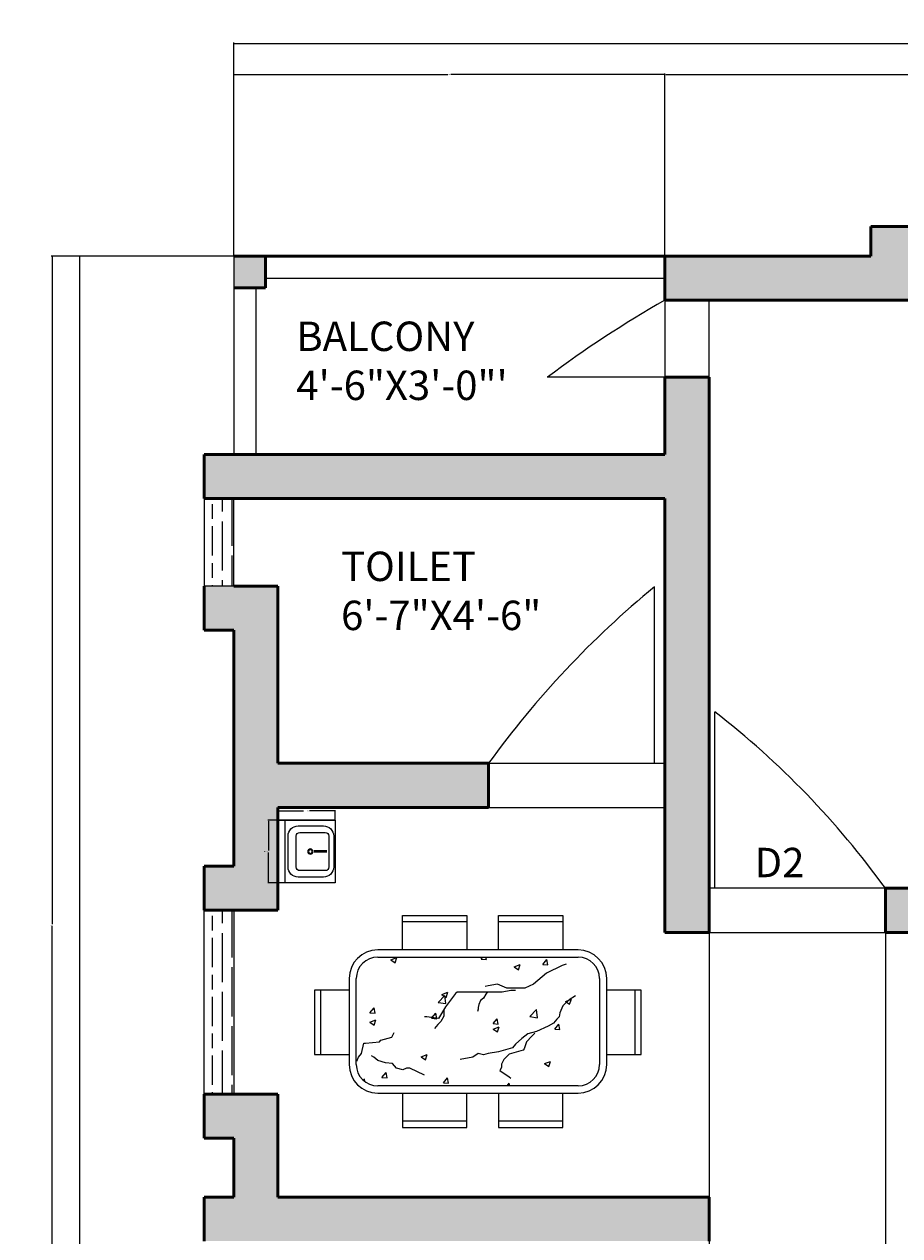
# Model space of a CAD drawing. Units: inches. Extents: x -12 to 604, y -566 to 58.
# Tile 5 of 12: x -12 to 166, y -189 to 58. Entities that reach past the tile are written whole.
import ezdxf

# ---------------------------------------------------------------- set-up
doc = ezdxf.new("R2010")
doc.units = ezdxf.units.IN
doc.header["$MEASUREMENT"] = 0
for name, color, linetype, lineweight in [('A-ANNO-DIMS', 2, 'Continuous', 18), ('A-ANNO-TEXT', 7, 'Continuous', 18), ('A-AREA-IDEN', 7, 'Continuous', 18), ('A-DOOR', 4, 'Continuous', 25), ('A-FLOR-FIXT', 9, 'Continuous', 18), ('A-FLOR-RAIL', 7, 'Continuous', 25), ('A-FURN', 8, 'Continuous', 18), ('A-GLAZ', 82, 'Continuous', 18), ('A-GLAZ-PATT', 82, 'Continuous', 13), ('A-WALL', 7, 'Continuous', 50), ('A-WALL-PATT', 18, 'Continuous', 13)]:
    doc.layers.add(name, color=color, linetype=linetype, lineweight=lineweight)
doc.styles.get("Standard").update_dxf_attribs({"font": 'arial.ttf'})
doc.dimstyles.get("Standard").update_dxf_attribs({"dimtxt": 0.18, "dimasz": 0.18, "dimexe": 0.18, "dimexo": 0.0625, "dimgap": 0.09, "dimtad": 0, "dimtih": 1, "dimtoh": 1, "dimdec": 0, "dimzin": 0, "dimdsep": 46, "dimlunit": 3, "dimtxsty": 'Standard', "dimcen": 0.09, "dimadec": 0, "dimazin": 0, "dimtfac": 1, "dimtdec": 0, "dimtofl": 0, "dimtmove": 0, "dimatfit": 3, "dimfxl": 1, "dimtolj": 1, "dimtzin": 0, "dimarcsym": 0})
pattern_1 = [(90, (0, 0), (6, -4e-16), [10, -2]), (90, (2, -2), (6, -4e-16), [6, -1.5, 3, -1.5]), (90, (4, -5), (6, -4e-16), [10, -2])]

# ---------------------------------------------------------------- blocks, each defined once
blk = doc.blocks.new('М14 600х655')
for p, q in [((-655, 600), (-655, 0)), ((-655, 600), (-655, 0)), ((-655, 0), (-655, 600)), ((0, 600), (-655, 600)), ((0, 525), (-655, 525)), ((0, 0), (0, 600)), ((-596, 388), (-596, 121)), ((-165, 494), (-490, 494)), ((-165, 408), (-490, 408)), ((-59, 121), (-59, 388)), ((-528, 370), (-528, 103)), ((-127, 103), (-127, 370)), ((-334, 87), (-334, 220)), ((-321, 87), (-321, 220)), ((-655, 0), (-655, 0)), ((-655, 0), (-655, 0)), ((-655, 0), (0, 0)), ((-655, 0), (0, 0)), ((-490, 65), (-165, 65)), ((-490, 15), (-165, 15))]:
    blk.add_line(p, q)
for radius in [27.6, 19.3]:
    blk.add_circle((-327, 259), radius)
for centre, radius, start, end in [((-490, 388), 106, 90, 180), ((-490, 370), 38.2, 90, 180), ((-165, 388), 106, 0, 90), ((-165, 370), 38.2, 0, 90), ((-490, 121), 106, 180, 270), ((-490, 103), 38.2, 180, 270), ((-165, 121), 106, 270, 0), ((-165, 103), 38.2, 270, 0)]:
    blk.add_arc(centre, radius, start, end)
blk = doc.blocks.new('*D4')
at = {"layer": 'A-ANNO-DIMS', "color": 0, "lineweight": -2, "transparency": 16777216}
for p, q in [((30.32, 11.2), (30.32, 54.68)), ((30.5, 54.5), (303.81, 54.5)), ((598.14, 54.5), (324.84, 54.5)), ((598.32, 11.2), (598.32, 54.68))]:
    blk.add_line(p, q, dxfattribs=at)
at = {"layer": 'A-ANNO-DIMS', "color": 0, "transparency": 16777216}
for points in [[(30.5, 54.53), (30.5, 54.47), (30.32, 54.5)], [(598.14, 54.53), (598.14, 54.47), (598.32, 54.5)]]:
    blk.add_solid(points, dxfattribs=at)
at = {"layer": 'Defpoints', "color": 0, "transparency": 16777216}
for p in [(598.32, 54.5), (30.32, 11.14), (598.32, 11.14)]:
    blk.add_point(p, dxfattribs=at)
at = {"layer": 'A-ANNO-DIMS', "color": 0, "transparency": 16777216, "insert": (314.32, 54.5), "char_height": 6, "attachment_point": 5}
blk.add_mtext('\\A1;47\'-4"', dxfattribs=at)
blk = doc.blocks.new('*D5')
at = {"layer": 'A-ANNO-DIMS', "color": 0, "lineweight": -2, "transparency": 16777216}
for p, q in [((30.26, 11.14), (-1.3, 11.14)), ((-1.12, 10.96), (-1.12, -233.2)), ((-1.12, -483.68), (-1.12, -239.51)), ((30.26, -483.86), (-1.3, -483.86))]:
    blk.add_line(p, q, dxfattribs=at)
at = {"layer": 'A-ANNO-DIMS', "color": 0, "transparency": 16777216}
for points in [[(-1.15, 10.96), (-1.09, 10.96), (-1.12, 11.14)], [(-1.15, -483.68), (-1.09, -483.68), (-1.12, -483.86)]]:
    blk.add_solid(points, dxfattribs=at)
at = {"layer": 'Defpoints', "color": 0, "transparency": 16777216}
for p in [(30.32, 11.14), (-1.12, -483.86), (30.32, -483.86)]:
    blk.add_point(p, dxfattribs=at)
at = {"layer": 'A-ANNO-DIMS', "color": 0, "transparency": 16777216, "insert": (-1.12, -236.36), "char_height": 6, "attachment_point": 5}
blk.add_mtext('\\A1;41\'-3"', dxfattribs=at)
blk = doc.blocks.new('DINING-TABLE-6-SEAT')
for p, q in [((17.93, 36.25), (17.93, 43.28)), ((17.93, 43.28), (31.08, 43.28)), ((31.08, 43.28), (31.08, 36.25)), ((37.5, 36.25), (37.5, 43.28)), ((37.5, 43.28), (50.64, 43.28)), ((50.64, 43.28), (50.64, 36.25)), ((31.08, 42), (17.93, 42)), ((50.64, 42), (37.5, 42)), ((53.77, 36.25), (12.88, 36.25)), ((12.88, 34.79), (53.77, 34.79)), ((15.53, 34.2), (16.76, 34.67)), ((16.41, 33.61), (16.76, 34.67)), ((34.01, 34.38), (34.34, 34.79)), ((35.05, 34.29), (34.96, 34.79)), ((15.53, 34.2), (16.41, 33.61)), ((34.01, 34.38), (35.05, 34.29)), ((40.72, 32.8), (41.94, 33.27)), ((40.72, 32.8), (41.59, 32.21)), ((41.59, 32.21), (41.95, 33.27)), ((46.57, 33.28), (47.42, 34.29)), ((46.57, 33.28), (47.62, 33.19)), ((50.53, 33.06), (47.35, 31.47)), ((47.62, 33.19), (47.42, 34.29)), ((51.32, 33.37), (50.53, 33.06)), ((7.04, 30.4), (7.04, 12.88)), ((8.5, 12.88), (8.5, 30.4)), ((47.35, 31.47), (44.66, 29.25)), ((58.15, 30.4), (58.15, 12.88)), ((59.61, 12.88), (59.61, 30.4)), ((0, 28.04), (0, 14.9)), ((7.04, 28.04), (0, 28.04)), ((1.29, 14.9), (1.29, 28.04)), ((25.99, 27.15), (27.22, 27.62)), ((28.78, 27.35), (26.71, 24.65)), ((26.87, 26.56), (27.22, 27.62)), ((29.09, 27.66), (28.78, 27.35)), ((38.3, 27.66), (29.09, 27.66)), ((35.45, 28.93), (34.81, 28.77)), ((35.29, 27.67), (34.97, 27.19)), ((37.35, 29.25), (35.45, 28.93)), ((39.26, 28.46), (37.35, 29.25)), ((40.05, 27.98), (38.3, 27.66)), ((42.91, 28.46), (39.26, 28.46)), ((41, 27.98), (40.05, 27.98)), ((44.66, 29.25), (42.91, 28.46)), ((66.65, 28.04), (59.61, 28.04)), ((65.37, 28.04), (65.37, 14.9)), ((66.65, 14.9), (66.65, 28.04)), ((25.21, 25.55), (26.57, 26.98)), ((25.21, 25.55), (26.76, 25.31)), ((25.99, 27.15), (26.87, 26.56)), ((26.76, 25.31), (26.57, 26.98)), ((33.54, 25.13), (33.38, 24.5)), ((33.86, 25.92), (33.54, 25.13)), ((34.49, 26.4), (33.86, 25.92)), ((34.97, 27.19), (34.49, 26.4)), ((50.69, 24.81), (50.05, 23.38)), ((51.96, 26.08), (50.69, 24.81)), ((51.18, 25.74), (52.41, 26.21)), ((51.18, 25.74), (52.05, 25.15)), ((53.23, 26.87), (51.96, 26.08)), ((52.05, 25.15), (52.41, 26.21)), ((11.3, 23.4), (12.14, 24.41)), ((11.3, 23.4), (12.35, 23.31)), ((12.35, 23.31), (12.14, 24.41)), ((22.9, 22.59), (22.42, 22.59)), ((25.28, 22.27), (22.9, 22.59)), ((23.87, 22.3), (24.71, 23.31)), ((23.87, 22.3), (24.91, 22.21)), ((24.92, 22.21), (24.71, 23.31)), ((26.71, 24.65), (25.28, 22.27)), ((26.39, 22.75), (25.76, 21.64)), ((26.39, 24.17), (26.39, 22.75)), ((33.38, 24.18), (33.22, 23.7)), ((33.38, 24.5), (33.38, 24.18)), ((43.91, 22.65), (45.27, 24.08)), ((43.91, 22.65), (45.47, 22.41)), ((45.47, 22.41), (45.27, 24.07)), ((49.9, 22.59), (49.42, 22.11)), ((50.05, 23.38), (49.9, 22.59)), ((11.27, 21.49), (12.5, 21.97)), ((11.27, 21.49), (12.14, 20.91)), ((12.14, 20.91), (12.5, 21.96)), ((25.12, 21), (24.49, 20.21)), ((25.76, 21.64), (25.12, 21)), ((36.44, 21.2), (37.28, 22.21)), ((36.44, 21.2), (37.48, 21.11)), ((36.45, 20.09), (37.68, 20.56)), ((36.45, 20.09), (37.33, 19.5)), ((37.48, 21.11), (37.28, 22.21)), ((37.33, 19.5), (37.68, 20.56)), ((47.67, 20.68), (45.29, 19.57)), ((48.78, 21.32), (47.67, 20.68)), ((49.42, 22.11), (48.78, 21.32)), ((49.01, 20.1), (49.85, 21.11)), ((49.01, 20.1), (50.05, 20.01)), ((50.05, 20.01), (49.85, 21.11)), ((10.36, 17.19), (13.21, 17.51)), ((13.21, 17.51), (13.53, 17.83)), ((13.53, 17.83), (15.76, 18.46)), ((15.76, 18.46), (16.23, 19.41)), ((42.27, 18.15), (41, 17.04)), ((43.54, 19.1), (42.27, 18.15)), ((43.23, 17.51), (42.75, 16.08)), ((44.34, 18.62), (43.23, 17.51)), ((45.29, 19.57), (43.54, 19.1)), ((44.97, 19.26), (44.34, 18.62)), ((0, 14.9), (7.04, 14.9)), ((8.93, 14.34), (9.56, 15.13)), ((9.56, 15.13), (10.04, 17.19)), ((10.04, 17.19), (10.36, 17.19)), ((21.73, 14.44), (22.96, 14.91)), ((22.6, 13.85), (22.96, 14.91)), ((33.38, 15.13), (32.27, 14.34)), ((34.49, 14.82), (33.38, 15.13)), ((35.45, 15.13), (34.49, 14.82)), ((37.51, 15.45), (35.45, 15.13)), ((40.37, 16.24), (37.51, 15.45)), ((39.73, 14.97), (38.62, 13.86)), ((42.59, 15.77), (39.73, 14.97)), ((41, 17.04), (40.37, 16.24)), ((42.75, 16.08), (42.59, 15.77)), ((59.61, 14.9), (66.65, 14.9)), ((8.61, 13.55), (8.93, 14.34)), ((12.11, 14.35), (11.63, 14.66)), ((12.9, 13.71), (12.11, 14.35)), ((14.49, 13.23), (12.9, 13.71)), ((15.92, 13.08), (14.49, 13.23)), ((16.71, 12.12), (15.92, 13.08)), ((21.73, 14.44), (22.6, 13.85)), ((32.27, 14.34), (29.73, 13.86)), ((38.62, 13.86), (38.14, 12.91)), ((38.14, 12.91), (38.14, 12.28)), ((46.91, 13.04), (48.14, 13.51)), ((46.91, 13.04), (47.79, 12.45)), ((47.79, 12.45), (48.14, 13.51)), ((9.93, 9.64), (10.19, 9.91)), ((10.25, 9.37), (10.19, 9.9)), ((13.73, 10.22), (14.57, 11.23)), ((13.73, 10.22), (14.78, 10.13)), ((14.78, 10.13), (14.57, 11.23)), ((17.98, 11.81), (16.71, 12.12)), ((18.77, 12.12), (17.98, 11.81)), ((19.41, 12.12), (18.77, 12.12)), ((22.43, 10.7), (19.41, 12.12)), ((26.3, 9.12), (27.14, 10.13)), ((27.35, 9.03), (27.14, 10.13)), ((38.14, 12.28), (37.83, 11.64)), ((37.83, 11.64), (39.73, 10.37)), ((39.73, 10.37), (40.05, 10.06)), ((53.77, 8.5), (12.88, 8.5)), ((26.3, 9.12), (27.35, 9.03)), ((39.27, 8.5), (39.71, 9.03)), ((39.81, 8.5), (39.71, 9.03)), ((12.88, 7.04), (53.77, 7.04)), ((17.93, 7.04), (17.93, 0)), ((31.08, 0), (31.08, 7.04)), ((37.5, 7.04), (37.5, 0)), ((50.64, 0), (50.64, 7.04)), ((31.08, 1.29), (17.93, 1.29)), ((50.64, 1.29), (37.5, 1.29)), ((17.93, 0), (31.08, 0)), ((37.5, 0), (50.64, 0))]:
    blk.add_line(p, q)
for centre, radius, start, end in [((12.88, 30.4), 5.84, 90, 180), ((12.88, 30.4), 4.38, 90, 180), ((53.77, 30.4), 5.84, 0, 90), ((53.77, 30.4), 4.38, 0, 90), ((12.88, 12.88), 5.84, 180, 270), ((12.88, 12.88), 4.38, 180, 270), ((53.77, 12.88), 4.38, 270, 0), ((53.77, 12.88), 5.84, 270, 0)]:
    blk.add_arc(centre, radius, start, end)
blk = doc.blocks.new('*D27')
at = {"layer": 'A-ANNO-DIMS', "color": 0, "lineweight": -2, "transparency": 16777216}
for p, q in [((39.28, -104), (37.25, -104)), ((37.43, -104.18), (37.43, -110.18)), ((37.43, -116.55), (37.43, -110.55)), ((39.28, -116.73), (37.25, -116.73))]:
    blk.add_line(p, q, dxfattribs=at)
at = {"layer": 'A-ANNO-DIMS', "color": 0, "transparency": 16777216}
for points in [[(37.4, -104.18), (37.46, -104.18), (37.43, -104)], [(37.4, -116.55), (37.46, -116.55), (37.43, -116.73)]]:
    blk.add_solid(points, dxfattribs=at)
at = {"layer": 'Defpoints', "color": 0, "transparency": 16777216}
for p in [(39.34, -104), (37.43, -116.73), (39.34, -116.73)]:
    blk.add_point(p, dxfattribs=at)
at = {"layer": 'A-ANNO-DIMS', "color": 0, "transparency": 16777216, "insert": (37.43, -110.36), "char_height": 0.18, "attachment_point": 5}
blk.add_mtext('\\A1;BASIN 1\'-0 1/2"', dxfattribs=at)
blk = doc.blocks.new('*D28')
at = {"layer": 'A-ANNO-DIMS', "color": 0, "lineweight": -2, "transparency": 16777216}
for p, q in [((39.34, -103.93), (39.34, -101.91)), ((39.52, -102.09), (44.56, -102.09)), ((50.83, -102.09), (45.78, -102.09)), ((51.01, -103.93), (51.01, -101.91))]:
    blk.add_line(p, q, dxfattribs=at)
at = {"layer": 'A-ANNO-DIMS', "color": 0, "transparency": 16777216}
for points in [[(39.52, -102.06), (39.52, -102.12), (39.34, -102.09)], [(50.83, -102.06), (50.83, -102.12), (51.01, -102.09)]]:
    blk.add_solid(points, dxfattribs=at)
at = {"layer": 'Defpoints', "color": 0, "transparency": 16777216}
for p in [(39.34, -102.09), (39.34, -104), (51.01, -104)]:
    blk.add_point(p, dxfattribs=at)
at = {"layer": 'A-ANNO-DIMS', "color": 0, "transparency": 16777216, "insert": (45.17, -102.09), "char_height": 0.18, "attachment_point": 5}
blk.add_mtext('\\A1;0\'-11 1/2"', dxfattribs=at)
blk = doc.blocks.new('*D51')
at = {"layer": 'A-ANNO-DIMS', "color": 0, "lineweight": -2, "transparency": 16777216}
for p, q in [((30.32, 11.2), (30.32, 48.37)), ((30.5, 48.19), (73.99, 48.19)), ((118.14, 48.19), (74.65, 48.19)), ((118.32, 11.2), (118.32, 48.37))]:
    blk.add_line(p, q, dxfattribs=at)
at = {"layer": 'A-ANNO-DIMS', "color": 0, "transparency": 16777216}
for points in [[(30.5, 48.22), (30.5, 48.16), (30.32, 48.19)], [(118.14, 48.22), (118.14, 48.16), (118.32, 48.19)]]:
    blk.add_solid(points, dxfattribs=at)
at = {"layer": 'Defpoints', "color": 0, "transparency": 16777216}
for p in [(118.32, 48.19), (30.32, 11.14), (118.32, 11.14)]:
    blk.add_point(p, dxfattribs=at)
at = {"layer": 'A-ANNO-DIMS', "color": 0, "transparency": 16777216, "insert": (74.32, 48.19), "char_height": 0.18, "attachment_point": 5}
blk.add_mtext('\\A1;7\'-4"', dxfattribs=at)
blk = doc.blocks.new('*D52')
at = {"layer": 'A-ANNO-DIMS', "color": 0, "lineweight": -2, "transparency": 16777216}
for p, q in [((118.32, 11.2), (118.32, 48.37)), ((118.5, 48.19), (198.93, 48.19)), ((280.14, 48.19), (199.71, 48.19)), ((280.32, 11.2), (280.32, 48.37))]:
    blk.add_line(p, q, dxfattribs=at)
at = {"layer": 'A-ANNO-DIMS', "color": 0, "transparency": 16777216}
for points in [[(118.5, 48.22), (118.5, 48.16), (118.32, 48.19)], [(280.14, 48.22), (280.14, 48.16), (280.32, 48.19)]]:
    blk.add_solid(points, dxfattribs=at)
at = {"layer": 'Defpoints', "color": 0, "transparency": 16777216}
for p in [(280.32, 48.19), (118.32, 11.14), (280.32, 11.14)]:
    blk.add_point(p, dxfattribs=at)
at = {"layer": 'A-ANNO-DIMS', "color": 0, "transparency": 16777216, "insert": (199.32, 48.19), "char_height": 0.18, "attachment_point": 5}
blk.add_mtext('\\A1;13\'-6"', dxfattribs=at)
blk = doc.blocks.new('*D54')
at = {"layer": 'A-ANNO-DIMS', "color": 0, "lineweight": -2, "transparency": 16777216}
for p, q in [((30.26, 11.14), (-6.91, 11.14)), ((-6.73, 10.96), (-6.73, -125.18)), ((-6.73, -261.68), (-6.73, -125.54)), ((39.26, -261.86), (-6.91, -261.86))]:
    blk.add_line(p, q, dxfattribs=at)
at = {"layer": 'A-ANNO-DIMS', "color": 0, "transparency": 16777216}
for points in [[(-6.76, 10.96), (-6.7, 10.96), (-6.73, 11.14)], [(-6.76, -261.68), (-6.7, -261.68), (-6.73, -261.86)]]:
    blk.add_solid(points, dxfattribs=at)
at = {"layer": 'Defpoints', "color": 0, "transparency": 16777216}
for p in [(30.32, 11.14), (-6.73, -261.86), (39.32, -261.86)]:
    blk.add_point(p, dxfattribs=at)
at = {"layer": 'A-ANNO-DIMS', "color": 0, "transparency": 16777216, "insert": (-6.73, -125.36), "char_height": 0.18, "attachment_point": 5}
blk.add_mtext('\\A1;22\'-9"', dxfattribs=at)
blk = doc.blocks.new('*D56')
at = {"layer": 'A-ANNO-DIMS', "color": 0, "lineweight": -2, "transparency": 16777216}
for p, q in [((127.32, -117.92), (127.32, -565.59)), ((163.32, -117.92), (163.32, -565.59)), ((127.5, -565.41), (144.99, -565.41)), ((163.14, -565.41), (145.65, -565.41))]:
    blk.add_line(p, q, dxfattribs=at)
at = {"layer": 'A-ANNO-DIMS', "color": 0, "transparency": 16777216}
for points in [[(127.5, -565.38), (127.5, -565.44), (127.32, -565.41)], [(163.14, -565.38), (163.14, -565.44), (163.32, -565.41)]]:
    blk.add_solid(points, dxfattribs=at)
at = {"layer": 'Defpoints', "color": 0, "transparency": 16777216}
for p in [(127.32, -117.86), (163.32, -117.86), (163.32, -565.41)]:
    blk.add_point(p, dxfattribs=at)
at = {"layer": 'A-ANNO-DIMS', "color": 0, "transparency": 16777216, "insert": (145.32, -565.41), "char_height": 0.18, "attachment_point": 5}
blk.add_mtext('\\A1;3\'-0"', dxfattribs=at)

msp = doc.modelspace()

# ---------------------------------------------------------------- hatches: boundary and pattern name
at = {"layer": 'A-GLAZ-PATT'}
h = msp.add_hatch(dxfattribs=at)
h.set_pattern_fill('GOST_WOOD', color=256)
h.set_pattern_definition(pattern_1)
h.paths.add_polyline_path([(30.32, -38.36), (24.32, -38.36), (24.32, -56.22), (30.32, -56.22)])
h = msp.add_hatch(dxfattribs=at)
h.set_pattern_fill('GOST_WOOD', color=256)
h.set_pattern_definition(pattern_1)
h.paths.add_polyline_path([(30.32, -122.36), (24.32, -122.36), (24.32, -159.86), (30.32, -159.86)])
at = {"layer": 'A-WALL-PATT'}
h = msp.add_hatch(color=256, dxfattribs=at)
h.dxf.hatch_style = 1
h.paths.add_polyline_path([(169.32, 11.14), (169.32, 17.14), (160.32, 17.14), (160.32, 11.14), (118.32, 11.14), (118.32, 6.64), (118.32, 2.14), (127.32, 2.14), (169.32, 2.14)])
h.paths.add_polyline_path([(127.32, -13.61), (118.32, -13.61), (118.32, -29.36), (34.82, -29.36), (24.32, -29.36), (24.32, -38.36), (39.32, -38.36), (118.32, -38.36), (118.32, -126.86), (127.32, -126.86), (127.32, -117.86)])
h.paths.add_polyline_path([(82.32, -92.36), (39.32, -92.36), (39.32, -56.22), (30.32, -56.22), (24.32, -56.22), (24.32, -65.22), (30.32, -65.22), (30.32, -113.36), (24.32, -113.36), (24.32, -122.36), (39.32, -122.36), (39.32, -101.36), (82.32, -101.36), (82.32, -96.86)], flags=17)
h.paths.add_polyline_path([(280.32, 11.14), (238.32, 11.14), (238.32, 17.14), (229.32, 17.14), (229.32, 12.64), (229.32, 11.14), (229.32, 2.14), (271.32, 2.14), (271.32, -117.86), (163.32, -117.86), (163.32, -126.86), (271.32, -126.86), (271.32, -189.86), (280.32, -189.86), (280.32, -180.86)])
h.paths.add_polyline_path([(415.32, 17.14), (406.32, 17.14), (406.32, 11.14), (358.32, 11.14), (358.32, -21.86), (367.32, -21.86), (367.32, 2.14), (415.32, 2.14)], flags=17)
h.paths.add_polyline_path([(484.55, -45.86), (448.32, -45.86), (448.32, 2.14), (448.32, 17.14), (439.32, 17.14), (439.32, 12.64), (439.32, 2.14), (439.32, -45.86), (367.32, -45.86), (358.32, -45.86), (358.32, -54.86), (430.32, -54.86), (430.32, -69.59), (430.32, -180.86), (318.82, -180.86), (318.82, -189.86), (318.82, -331.86), (327.82, -331.86), (327.82, -189.86), (439.32, -189.86), (439.32, -180.86), (439.32, -54.86), (483.5, -54.86), (484.55, -54.86)])
h.paths.add_polyline_path([(529.32, 11.14), (481.32, 11.14), (481.32, 17.14), (472.32, 17.14), (472.32, 12.64), (472.32, 2.14), (520.32, 2.14), (520.32, -21.86), (529.32, -21.86)])
h.paths.add_polyline_path([(598.32, -45.86), (582.42, -45.86), (582.42, -50.36), (582.42, -54.86), (589.32, -54.86), (589.32, -99.86), (598.32, -99.86), (604.32, -99.86), (604.32, -90.86), (598.32, -90.86)])
h.paths.add_polyline_path([(598.32, -168.86), (604.32, -168.86), (604.32, -159.86), (589.32, -159.86), (589.32, -180.86), (477.32, -180.86), (477.32, -189.86), (477.32, -259.86), (486.32, -259.86), (486.32, -189.86), (589.32, -189.86), (589.32, -204.86), (598.32, -204.86), (604.32, -204.86), (604.32, -195.86), (598.32, -195.86)])
h.paths.add_polyline_path([(598.32, -244.86), (604.32, -244.86), (604.32, -235.86), (598.32, -235.86), (589.32, -235.86), (589.32, -250.86), (522.32, -250.86), (522.32, -259.86), (589.32, -259.86), (589.32, -274.86), (598.32, -274.86), (604.32, -274.86), (604.32, -265.86), (598.32, -265.86)])
h.paths.add_polyline_path([(598.32, -333.28), (604.32, -333.28), (604.32, -324.28), (598.32, -324.28), (598.32, -321.87), (598.32, -318.28), (604.32, -318.28), (604.32, -309.28), (598.32, -309.28), (589.32, -309.28), (589.32, -341.95), (589.38, -341.95), (589.38, -363.16), (589.32, -381.86), (565.32, -381.86), (565.32, -390.86), (589.32, -390.86), (589.32, -450.86), (598.32, -450.86), (604.32, -450.86), (604.32, -441.86), (598.32, -441.86), (598.32, -390.86), (604.32, -390.86), (604.32, -381.86), (598.32, -381.86)])
h.paths.add_polyline_path([(541.32, -345.86), (424.32, -345.86), (424.32, -354.86), (532.32, -354.86), (532.32, -474.86), (463.39, -474.86), (463.39, -483.86), (553.32, -483.86), (553.32, -474.86), (541.32, -474.86), (541.32, -390.86), (541.32, -381.86)])
h.paths.add_polyline_path([(604.32, -474.86), (589.32, -474.86), (553.32, -474.86), (553.32, -483.86), (598.32, -483.86), (604.32, -483.86)])
h.paths.add_polyline_path([(388.32, -483.86), (388.32, -474.86), (388.32, -460.13), (388.32, -333.86), (388.32, -322.86), (379.32, -322.86), (379.32, -331.86), (379.32, -333.86), (379.32, -474.86), (379.32, -520.86), (344.32, -520.86), (344.32, -529.86), (379.32, -529.86), (388.32, -529.86)])
h.paths.add_polyline_path([(284.32, -520.86), (249.32, -520.86), (249.32, -474.86), (249.32, -368.36), (240.32, -368.36), (240.32, -474.86), (238.52, -474.86), (238.52, -483.86), (240.32, -483.86), (240.32, -529.86), (249.32, -529.86), (284.32, -529.86)])
h.paths.add_polyline_path([(178.82, -474.86), (158.91, -474.86), (158.91, -483.86), (162.32, -483.86), (178.82, -483.86)])
h.paths.add_polyline_path([(84.32, -474.86), (84.32, -366.86), (75.32, -366.86), (75.32, -474.86), (39.32, -474.86), (39.32, -453.86), (24.32, -453.86), (24.32, -462.86), (30.32, -462.86), (30.32, -483.86), (84.32, -483.86)])
h.paths.add_polyline_path([(39.32, -342.86), (75.32, -342.86), (84.32, -342.86), (179.67, -342.86), (179.67, -333.86), (39.32, -333.86), (39.32, -318.86), (24.32, -318.86), (24.32, -327.86), (30.32, -327.86), (30.32, -432.86), (24.32, -432.86), (24.32, -441.86), (30.32, -441.86), (39.32, -441.86)])
h.paths.add_polyline_path([(249.32, -252.86), (115.32, -252.86), (115.32, -225.86), (106.32, -225.86), (106.32, -252.86), (39.32, -252.86), (39.32, -237.86), (24.32, -237.86), (24.32, -246.86), (30.32, -246.86), (30.32, -267.86), (24.32, -267.86), (24.32, -276.86), (39.32, -276.86), (39.32, -261.86), (240.32, -261.86), (240.32, -331.86), (249.32, -331.86), (266.82, -331.86), (266.82, -322.86), (249.32, -322.86)])
h.paths.add_polyline_path([(127.32, -180.86), (39.32, -180.86), (24.32, -180.86), (24.32, -189.86), (39.32, -189.86), (127.32, -189.86)])
h.paths.add_polyline_path([(39.32, -159.86), (24.32, -159.86), (24.32, -168.86), (30.32, -168.86), (30.32, -180.86), (39.32, -180.86)])
h.paths.add_polyline_path([(470.51, -17.27), (512.48, -17.27), (512.48, 5.12), (470.51, 5.12)], flags=9)
h.paths.add_polyline_path([(484.21, -244.26), (526.45, -244.26), (526.45, -221.87), (484.21, -221.87)], flags=24)
h.paths.add_polyline_path([(36.91, -442.88), (83.54, -442.88), (83.54, -420.5), (36.91, -420.5)], flags=25)
h = msp.add_hatch(color=256, dxfattribs=at)
h.dxf.hatch_style = 1
h.paths.add_polyline_path([(598.32, 11.14), (591.82, 11.14), (591.82, 6.64), (593.82, 6.64), (593.82, 4.64), (598.32, 4.64)])
h.paths.add_polyline_path([(36.82, 6.64), (36.82, 11.14), (30.32, 11.14), (30.32, 4.64), (34.82, 4.64), (36.82, 4.64)])

# ---------------------------------------------------------------- linework, layer by layer
at = {"layer": 'A-DOOR'}
for p, q in [((118.32, 2.14), (118.32, -13.61)), ((127.32, 2.14), (118.32, 2.14)), ((127.32, -13.61), (127.32, 2.14)), ((118.32, -13.61), (94.32, -13.61)), ((118.32, -13.61), (127.32, -13.61)), ((116.19, -92.36), (116.19, -56.36)), ((128.52, -117.86), (128.52, -81.86)), ((82.32, -92.36), (118.32, -92.36)), ((82.32, -92.36), (82.32, -96.86)), ((118.32, -101.36), (118.32, -92.36)), ((82.32, -96.86), (82.32, -101.36)), ((82.32, -101.36), (118.32, -101.36)), ((163.32, -117.86), (127.32, -117.86)), ((127.32, -117.86), (127.32, -126.86)), ((163.32, -126.86), (163.32, -117.86)), ((127.32, -126.86), (163.32, -126.86))]:
    msp.add_line(p, q, dxfattribs=at)
for centre, radius, start, end in [((232.03, -197.28), 229.56, 119.6902, 126.8596), ((238.97, -205.79), 193.4, 129.4079, 144.0908), ((19.69, -221.88), 177.34, 35.9132, 52.1438)]:
    msp.add_arc(centre, radius, start, end, dxfattribs=at)
at = {"layer": 'A-FLOR-RAIL'}
for p, q in [((30.32, 11.14), (30.32, -29.36)), ((36.82, 6.64), (118.32, 6.64)), ((34.82, 4.64), (34.82, -29.36))]:
    msp.add_line(p, q, dxfattribs=at)
at = {"layer": 'A-GLAZ'}
for p, q in [((24.32, -38.36), (24.32, -56.22)), ((30.32, -56.22), (30.32, -38.36)), ((30.32, -56.22), (24.32, -56.22)), ((24.32, -159.86), (24.32, -122.36)), ((30.32, -122.36), (30.32, -159.86))]:
    msp.add_line(p, q, dxfattribs=at)
at = {"layer": 'A-WALL'}
for p, q in [((160.32, 17.14), (169.32, 17.14)), ((160.32, 11.14), (160.32, 17.14)), ((30.32, 11.14), (160.32, 11.14)), ((36.82, 6.64), (36.82, 11.14)), ((118.32, 6.64), (118.32, 11.14)), ((36.82, 4.64), (36.82, 6.64)), ((118.32, 6.64), (118.32, 2.14)), ((34.82, 4.64), (30.32, 4.64)), ((34.82, 4.64), (36.82, 4.64)), ((127.32, 2.14), (118.32, 2.14)), ((127.32, 2.14), (169.32, 2.14)), ((122.82, -13.61), (118.32, -13.61)), ((118.32, -13.61), (118.32, -29.36)), ((122.82, -13.61), (127.32, -13.61)), ((127.32, -13.61), (127.32, -117.86)), ((24.32, -38.36), (24.32, -29.36)), ((24.32, -29.36), (34.82, -29.36)), ((34.82, -29.36), (118.32, -29.36)), ((39.32, -38.36), (24.32, -38.36)), ((39.32, -38.36), (118.32, -38.36)), ((118.32, -38.36), (118.32, -126.86)), ((24.32, -65.22), (24.32, -56.22)), ((30.32, -56.22), (39.32, -56.22)), ((39.32, -56.22), (39.32, -92.36)), ((30.32, -65.22), (24.32, -65.22)), ((30.32, -65.22), (30.32, -113.36)), ((39.32, -92.36), (82.32, -92.36)), ((82.32, -92.36), (82.32, -101.36)), ((39.32, -101.36), (82.32, -101.36)), ((39.32, -101.36), (39.32, -122.36)), ((30.32, -113.36), (24.32, -113.36)), ((24.32, -122.36), (24.32, -113.36)), ((127.32, -117.86), (127.32, -126.86)), ((163.32, -117.86), (271.32, -117.86)), ((163.32, -126.86), (163.32, -117.86)), ((24.32, -122.36), (39.32, -122.36)), ((118.32, -126.86), (127.32, -126.86)), ((163.32, -126.86), (271.32, -126.86)), ((24.32, -159.86), (39.32, -159.86)), ((24.32, -168.86), (24.32, -159.86)), ((39.32, -159.86), (39.32, -180.86)), ((30.32, -168.86), (24.32, -168.86)), ((30.32, -168.86), (30.32, -180.86)), ((30.32, -180.86), (24.32, -180.86)), ((24.32, -189.86), (24.32, -180.86)), ((39.32, -180.86), (127.32, -180.86)), ((127.32, -180.86), (127.32, -189.86))]:
    msp.add_line(p, q, dxfattribs=at)

# ---------------------------------------------------------------- block references
at = {"layer": 'A-FLOR-FIXT', "xscale": -0.0194421461217856, "yscale": 0.0194421461217856, "zscale": 0.0194421461217856, "rotation": 90}
msp.add_blockref('М14 600х655', (51.01, -116.73), dxfattribs=at)
at = {"layer": 'A-FURN'}
msp.add_blockref('DINING-TABLE-6-SEAT', (46.83, -166.69), dxfattribs=at)

# ---------------------------------------------------------------- texts
at = {"layer": 'A-ANNO-TEXT', "insert": (136.61, -109.61), "char_height": 6, "attachment_point": 1}
msp.add_mtext('D2', dxfattribs=at)
at = {"layer": 'A-AREA-IDEN', "insert": (43.1, -2.24), "char_height": 6, "attachment_point": 1}
msp.add_mtext_dynamic_manual_height_columns('BALCONY\\P4\'-6"X3\'-0"\'', width=0.1877, gutter_width=1, heights=[0], dxfattribs=at)
at = {"layer": 'A-AREA-IDEN', "insert": (52.23, -49.18), "char_height": 6, "attachment_point": 1}
msp.add_mtext('TOILET\\P6\'-7"X4\'-6"', dxfattribs=at)

# ---------------------------------------------------------------- dimensions: what is measured, and where the dimension line sits
at = {"layer": 'A-ANNO-DIMS'}
for base, p1, p2, override, picture, middle in [((598.32, 54.5), (30.32, 11.14), (598.32, 11.14), {"dimtxt": 6, "dimclrd": 0, "dimclre": 0, "dimclrt": 0}, '*D4', (314.32, 54.5)), ((118.32, 48.19), (30.32, 11.14), (118.32, 11.14), {"dimdec": 1, "dimlfac": 1, "dimrnd": 0, "dimzin": 1, "dimdsep": 46, "dimlunit": 4, "dimfrac": 2}, '*D51', (74.32, 48.19)), ((280.32, 48.19), (118.32, 11.14), (280.32, 11.14), {"dimdec": 1, "dimlfac": 1, "dimrnd": 0, "dimzin": 1, "dimdsep": 46, "dimlunit": 4, "dimfrac": 2}, '*D52', (199.32, 48.19)), ((163.32, -565.41), (127.32, -117.86), (163.32, -117.86), {"dimdec": 1, "dimlfac": 1, "dimrnd": 0, "dimzin": 1, "dimdsep": 46, "dimlunit": 4, "dimfrac": 2}, '*D56', (145.32, -565.41))]:
    dim = msp.add_linear_dim(base=base, p1=p1, p2=p2, dimstyle='Standard', override=override, dxfattribs=at)
    dim.commit()
    dim.dimension.update_dxf_attribs({"geometry": picture, "text_midpoint": middle})
for base, p1, p2, angle, override, picture, middle in [((-1.12, -483.86), (30.32, 11.14), (30.32, -483.86), 90, {"dimtxt": 6, "dimclrd": 0, "dimclre": 0, "dimclrt": 0}, '*D5', (-1.12, -236.36)), ((-6.73, -261.86), (30.32, 11.14), (39.32, -261.86), 90, {"dimdec": 1, "dimlfac": 1, "dimrnd": 0, "dimzin": 1, "dimdsep": 46, "dimlunit": 4, "dimfrac": 2}, '*D54', (-6.73, -125.36)), ((39.34, -102.09), (51.01, -104), (39.34, -104), 180, {"dimdec": 1, "dimlfac": 1, "dimrnd": 0, "dimzin": 1, "dimdsep": 46, "dimlunit": 4, "dimfrac": 2}, '*D28', (45.17, -102.09))]:
    dim = msp.add_linear_dim(base=base, p1=p1, p2=p2, angle=angle, dimstyle='Standard', override=override, dxfattribs=at)
    dim.commit()
    dim.dimension.update_dxf_attribs({"geometry": picture, "text_midpoint": middle})
dim = msp.add_linear_dim(base=(37.43, -116.73), p1=(39.34, -104), p2=(39.34, -116.73), angle=270, text='BASIN <>', dimstyle='Standard', override={"dimdec": 1, "dimlfac": 1, "dimrnd": 0, "dimzin": 1, "dimdsep": 46, "dimlunit": 4, "dimfrac": 2}, dxfattribs=at)
dim.commit()
dim.dimension.update_dxf_attribs({"geometry": '*D27', "text_midpoint": (37.43, -110.36)})

doc.saveas('drawing.dxf')
